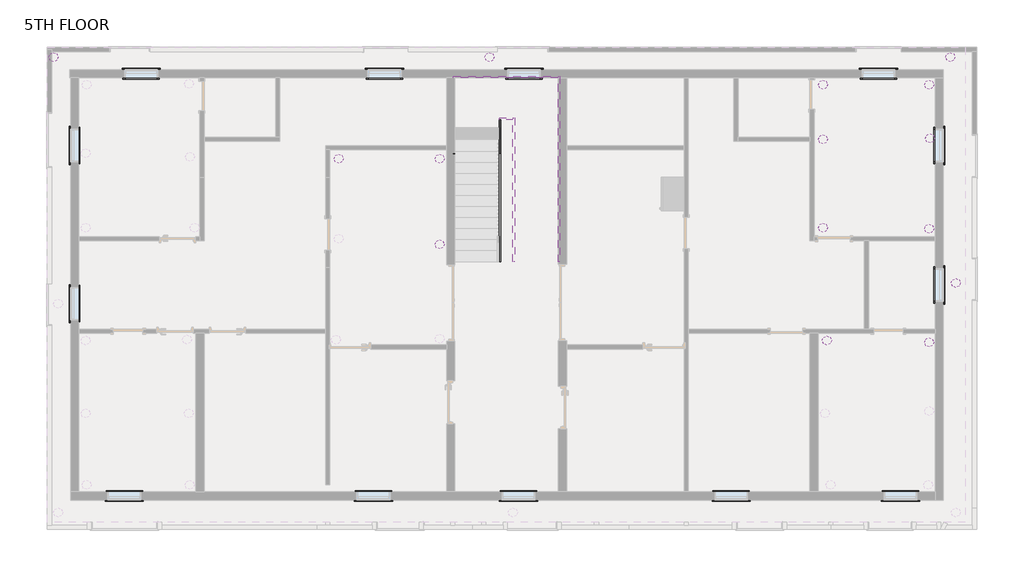
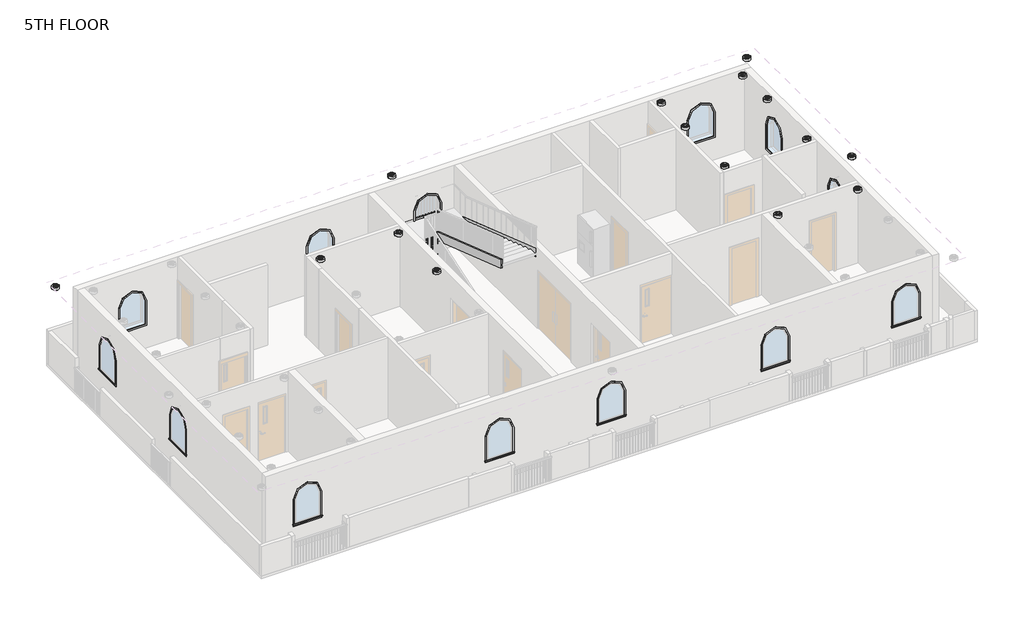
# One storey, part 7 of 7: 26 proxies, 15 light fixtures, 6 members.
"""IFC4 building model written with IfcOpenShell, lengths in millimetres."""

from ifc_helpers import new_model, si_unit, frame, origin, place, context, project, spatial, polyline, outline, extrude, transform, mapped, element, save
from components import trim_window_exterior_flat_arch_top_tree_centered_with_sill_aed3e54d, trim_window_interior_flat_arch_top_tree_centered_picture_e2e46177, ceiling_light_flat_round_60w_120v_7c4c2a52

model = new_model("IFC4")

# Units and contexts
model_context = context("Model", 3, world=origin())
ifc_project = project(units=[si_unit("LENGTHUNIT", "METRE", prefix="MILLI")], contexts=[model_context])

# Site, building, storey
site = spatial("IfcSite", under=ifc_project)
building = spatial("IfcBuilding", under=site)
storey = spatial("IfcBuildingStorey", under=building, Name="5TH FLOOR", Elevation=16002.0)

# Proxies
placement = place(None, origin())
trim_window_exterior_flat_arch_top_tree_centered_with_sill_shape = trim_window_exterior_flat_arch_top_tree_centered_with_sill_aed3e54d(model_context)
element("IfcBuildingElementProxy", 1, Name="Trim-Window-Exterior-Flat-Arch-Top-Tree_Centered : with Sill", ObjectType="Trim-Window-Exterior-Flat-Arch-Top-Tree_Centered : with Sill", at=placement, inside=storey, context=model_context, shape_type="MappedRepresentation", body=[
    mapped(trim_window_exterior_flat_arch_top_tree_centered_with_sill_shape, transform((-10967.3987925, -4014.0932193, 18288.0), x_axis=(1.0, 0.0, 0.0), y_axis=(0.0, 0.0, 1.0), z_axis=(0.0, -1.0, 0.0))),
])
element("IfcBuildingElementProxy", 2, Name="Trim-Window-Exterior-Flat-Arch-Top-Tree_Centered : with Sill", ObjectType="Trim-Window-Exterior-Flat-Arch-Top-Tree_Centered : with Sill", at=placement, inside=storey, context=model_context, shape_type="MappedRepresentation", body=[
    mapped(trim_window_exterior_flat_arch_top_tree_centered_with_sill_shape, transform((-4096.6987998, -4014.0932193, 18288.0), x_axis=(1.0, 0.0, 0.0), y_axis=(0.0, 0.0, 1.0), z_axis=(0.0, -1.0, 0.0))),
])
element("IfcBuildingElementProxy", 3, Name="Trim-Window-Exterior-Flat-Arch-Top-Tree_Centered : with Sill", ObjectType="Trim-Window-Exterior-Flat-Arch-Top-Tree_Centered : with Sill", at=placement, inside=storey, context=model_context, shape_type="MappedRepresentation", body=[
    mapped(trim_window_exterior_flat_arch_top_tree_centered_with_sill_shape, transform((-96.7067989, -4014.0932193, 18288.0), x_axis=(1.0, 0.0, 0.0), y_axis=(0.0, 0.0, 1.0), z_axis=(0.0, -1.0, 0.0))),
])
element("IfcBuildingElementProxy", 4, Name="Trim-Window-Exterior-Flat-Arch-Top-Tree_Centered : with Sill", ObjectType="Trim-Window-Exterior-Flat-Arch-Top-Tree_Centered : with Sill", at=placement, inside=storey, context=model_context, shape_type="MappedRepresentation", body=[
    mapped(trim_window_exterior_flat_arch_top_tree_centered_with_sill_shape, transform((5771.2012079, -4014.0932193, 18288.0), x_axis=(1.0, 0.0, 0.0), y_axis=(0.0, 0.0, 1.0), z_axis=(0.0, -1.0, 0.0))),
])
element("IfcBuildingElementProxy", 5, Name="Trim-Window-Exterior-Flat-Arch-Top-Tree_Centered : with Sill", ObjectType="Trim-Window-Exterior-Flat-Arch-Top-Tree_Centered : with Sill", at=placement, inside=storey, context=model_context, shape_type="MappedRepresentation", body=[
    mapped(trim_window_exterior_flat_arch_top_tree_centered_with_sill_shape, transform((10444.8012075, -4014.0932193, 18288.0), x_axis=(1.0, 0.0, 0.0), y_axis=(0.0, 0.0, 1.0), z_axis=(0.0, -1.0, 0.0))),
])
element("IfcBuildingElementProxy", 6, Name="Trim-Window-Exterior-Flat-Arch-Top-Tree_Centered : with Sill", ObjectType="Trim-Window-Exterior-Flat-Arch-Top-Tree_Centered : with Sill", at=placement, inside=storey, context=model_context, shape_type="MappedRepresentation", body=[
    mapped(trim_window_exterior_flat_arch_top_tree_centered_with_sill_shape, transform((11625.9012075, 1916.8067333, 18288.0), x_axis=(0.0, 1.0, 0.0), y_axis=(0.0, 0.0, 1.0), z_axis=(1.0, 0.0, 0.0))),
])
element("IfcBuildingElementProxy", 7, Name="Trim-Window-Exterior-Flat-Arch-Top-Tree_Centered : with Sill", ObjectType="Trim-Window-Exterior-Flat-Arch-Top-Tree_Centered : with Sill", at=placement, inside=storey, context=model_context, shape_type="MappedRepresentation", body=[
    mapped(trim_window_exterior_flat_arch_top_tree_centered_with_sill_shape, transform((11625.9012075, 5764.9067329, 18288.0), x_axis=(0.0, 1.0, 0.0), y_axis=(0.0, 0.0, 1.0), z_axis=(1.0, 0.0, 0.0))),
])
element("IfcBuildingElementProxy", 8, Name="Trim-Window-Exterior-Flat-Arch-Top-Tree_Centered : with Sill", ObjectType="Trim-Window-Exterior-Flat-Arch-Top-Tree_Centered : with Sill", at=placement, inside=storey, context=model_context, shape_type="MappedRepresentation", body=[
    mapped(trim_window_exterior_flat_arch_top_tree_centered_with_sill_shape, transform((9835.2012075, 7860.4067329, 18288.0), x_axis=(-1.0, 0.0, 0.0), y_axis=(0.0, 0.0, 1.0), z_axis=(0.0, 1.0, 0.0))),
])
element("IfcBuildingElementProxy", 9, Name="Trim-Window-Exterior-Flat-Arch-Top-Tree_Centered : with Sill", ObjectType="Trim-Window-Exterior-Flat-Arch-Top-Tree_Centered : with Sill", at=placement, inside=storey, context=model_context, shape_type="MappedRepresentation", body=[
    mapped(trim_window_exterior_flat_arch_top_tree_centered_with_sill_shape, transform((55.6932011, 7860.4067329, 18288.0), x_axis=(-1.0, 0.0, 0.0), y_axis=(0.0, 0.0, 1.0), z_axis=(0.0, 1.0, 0.0))),
])
element("IfcBuildingElementProxy", 10, Name="Trim-Window-Exterior-Flat-Arch-Top-Tree_Centered : with Sill", ObjectType="Trim-Window-Exterior-Flat-Arch-Top-Tree_Centered : with Sill", at=placement, inside=storey, context=model_context, shape_type="MappedRepresentation", body=[
    mapped(trim_window_exterior_flat_arch_top_tree_centered_with_sill_shape, transform((-3791.8987998, 7860.4067329, 18288.0), x_axis=(-1.0, 0.0, 0.0), y_axis=(0.0, 0.0, 1.0), z_axis=(0.0, 1.0, 0.0))),
])
element("IfcBuildingElementProxy", 11, Name="Trim-Window-Exterior-Flat-Arch-Top-Tree_Centered : with Sill", ObjectType="Trim-Window-Exterior-Flat-Arch-Top-Tree_Centered : with Sill", at=placement, inside=storey, context=model_context, shape_type="MappedRepresentation", body=[
    mapped(trim_window_exterior_flat_arch_top_tree_centered_with_sill_shape, transform((-10503.8487992, 7860.4067329, 18288.0), x_axis=(-1.0, 0.0, 0.0), y_axis=(0.0, 0.0, 1.0), z_axis=(0.0, 1.0, 0.0))),
])
element("IfcBuildingElementProxy", 12, Name="Trim-Window-Exterior-Flat-Arch-Top-Tree_Centered : with Sill", ObjectType="Trim-Window-Exterior-Flat-Arch-Top-Tree_Centered : with Sill", at=placement, inside=storey, context=model_context, shape_type="MappedRepresentation", body=[
    mapped(trim_window_exterior_flat_arch_top_tree_centered_with_sill_shape, transform((-12453.2987925, 5764.9067329, 18288.0), x_axis=(0.0, -1.0, 0.0), y_axis=(0.0, 0.0, 1.0), z_axis=(-1.0, 0.0, 0.0))),
])
element("IfcBuildingElementProxy", 13, Name="Trim-Window-Exterior-Flat-Arch-Top-Tree_Centered : with Sill", ObjectType="Trim-Window-Exterior-Flat-Arch-Top-Tree_Centered : with Sill", at=placement, inside=storey, context=model_context, shape_type="MappedRepresentation", body=[
    mapped(trim_window_exterior_flat_arch_top_tree_centered_with_sill_shape, transform((-12453.2987925, 1402.4567334, 18288.0), x_axis=(0.0, -1.0, 0.0), y_axis=(0.0, 0.0, 1.0), z_axis=(-1.0, 0.0, 0.0))),
])
trim_window_interior_flat_arch_top_tree_centered_picture_shape = trim_window_interior_flat_arch_top_tree_centered_picture_e2e46177(model_context)
element("IfcBuildingElementProxy", 14, Name="Trim-Window-Interior-Flat-Arch-Top-Tree_Centered : Picture Frame", ObjectType="Trim-Window-Interior-Flat-Arch-Top-Tree_Centered : Picture Frame", at=placement, inside=storey, context=model_context, shape_type="MappedRepresentation", body=[
    mapped(trim_window_interior_flat_arch_top_tree_centered_picture_shape, transform((-10967.3987925, -3785.4932193, 18288.0), x_axis=(-1.0, 0.0, 0.0), y_axis=(0.0, 0.0, 1.0), z_axis=(0.0, 1.0, 0.0))),
])
element("IfcBuildingElementProxy", 15, Name="Trim-Window-Interior-Flat-Arch-Top-Tree_Centered : Picture Frame", ObjectType="Trim-Window-Interior-Flat-Arch-Top-Tree_Centered : Picture Frame", at=placement, inside=storey, context=model_context, shape_type="MappedRepresentation", body=[
    mapped(trim_window_interior_flat_arch_top_tree_centered_picture_shape, transform((-4096.6987998, -3785.4932193, 18288.0), x_axis=(-1.0, 0.0, 0.0), y_axis=(0.0, 0.0, 1.0), z_axis=(0.0, 1.0, 0.0))),
])
element("IfcBuildingElementProxy", 16, Name="Trim-Window-Interior-Flat-Arch-Top-Tree_Centered : Picture Frame", ObjectType="Trim-Window-Interior-Flat-Arch-Top-Tree_Centered : Picture Frame", at=placement, inside=storey, context=model_context, shape_type="MappedRepresentation", body=[
    mapped(trim_window_interior_flat_arch_top_tree_centered_picture_shape, transform((-96.7067989, -3785.4932193, 18288.0), x_axis=(-1.0, 0.0, 0.0), y_axis=(0.0, 0.0, 1.0), z_axis=(0.0, 1.0, 0.0))),
])
element("IfcBuildingElementProxy", 17, Name="Trim-Window-Interior-Flat-Arch-Top-Tree_Centered : Picture Frame", ObjectType="Trim-Window-Interior-Flat-Arch-Top-Tree_Centered : Picture Frame", at=placement, inside=storey, context=model_context, shape_type="MappedRepresentation", body=[
    mapped(trim_window_interior_flat_arch_top_tree_centered_picture_shape, transform((5771.2012079, -3785.4932193, 18288.0), x_axis=(-1.0, 0.0, 0.0), y_axis=(0.0, 0.0, 1.0), z_axis=(0.0, 1.0, 0.0))),
])
element("IfcBuildingElementProxy", 18, Name="Trim-Window-Interior-Flat-Arch-Top-Tree_Centered : Picture Frame", ObjectType="Trim-Window-Interior-Flat-Arch-Top-Tree_Centered : Picture Frame", at=placement, inside=storey, context=model_context, shape_type="MappedRepresentation", body=[
    mapped(trim_window_interior_flat_arch_top_tree_centered_picture_shape, transform((10444.8012075, -3785.4932193, 18288.0), x_axis=(-1.0, 0.0, 0.0), y_axis=(0.0, 0.0, 1.0), z_axis=(0.0, 1.0, 0.0))),
])
element("IfcBuildingElementProxy", 19, Name="Trim-Window-Interior-Flat-Arch-Top-Tree_Centered : Picture Frame", ObjectType="Trim-Window-Interior-Flat-Arch-Top-Tree_Centered : Picture Frame", at=placement, inside=storey, context=model_context, shape_type="MappedRepresentation", body=[
    mapped(trim_window_interior_flat_arch_top_tree_centered_picture_shape, transform((11397.3012075, 1916.8067333, 18288.0), x_axis=(0.0, -1.0, 0.0), y_axis=(0.0, 0.0, 1.0), z_axis=(-1.0, 0.0, 0.0))),
])
element("IfcBuildingElementProxy", 20, Name="Trim-Window-Interior-Flat-Arch-Top-Tree_Centered : Picture Frame", ObjectType="Trim-Window-Interior-Flat-Arch-Top-Tree_Centered : Picture Frame", at=placement, inside=storey, context=model_context, shape_type="MappedRepresentation", body=[
    mapped(trim_window_interior_flat_arch_top_tree_centered_picture_shape, transform((11397.3012075, 5764.9067329, 18288.0), x_axis=(0.0, -1.0, 0.0), y_axis=(0.0, 0.0, 1.0), z_axis=(-1.0, 0.0, 0.0))),
])
element("IfcBuildingElementProxy", 21, Name="Trim-Window-Interior-Flat-Arch-Top-Tree_Centered : Picture Frame", ObjectType="Trim-Window-Interior-Flat-Arch-Top-Tree_Centered : Picture Frame", at=placement, inside=storey, context=model_context, shape_type="MappedRepresentation", body=[
    mapped(trim_window_interior_flat_arch_top_tree_centered_picture_shape, transform((9835.2012075, 7631.8067329, 18288.0), x_axis=(1.0, 0.0, 0.0), y_axis=(0.0, 0.0, 1.0), z_axis=(0.0, -1.0, 0.0))),
])
element("IfcBuildingElementProxy", 22, Name="Trim-Window-Interior-Flat-Arch-Top-Tree_Centered : Picture Frame", ObjectType="Trim-Window-Interior-Flat-Arch-Top-Tree_Centered : Picture Frame", at=placement, inside=storey, context=model_context, shape_type="MappedRepresentation", body=[
    mapped(trim_window_interior_flat_arch_top_tree_centered_picture_shape, transform((55.6932011, 7631.8067329, 18288.0), x_axis=(1.0, 0.0, 0.0), y_axis=(0.0, 0.0, 1.0), z_axis=(0.0, -1.0, 0.0))),
])
element("IfcBuildingElementProxy", 23, Name="Trim-Window-Interior-Flat-Arch-Top-Tree_Centered : Picture Frame", ObjectType="Trim-Window-Interior-Flat-Arch-Top-Tree_Centered : Picture Frame", at=placement, inside=storey, context=model_context, shape_type="MappedRepresentation", body=[
    mapped(trim_window_interior_flat_arch_top_tree_centered_picture_shape, transform((-3791.8987998, 7631.8067329, 18288.0), x_axis=(1.0, 0.0, 0.0), y_axis=(0.0, 0.0, 1.0), z_axis=(0.0, -1.0, 0.0))),
])
element("IfcBuildingElementProxy", 24, Name="Trim-Window-Interior-Flat-Arch-Top-Tree_Centered : Picture Frame", ObjectType="Trim-Window-Interior-Flat-Arch-Top-Tree_Centered : Picture Frame", at=placement, inside=storey, context=model_context, shape_type="MappedRepresentation", body=[
    mapped(trim_window_interior_flat_arch_top_tree_centered_picture_shape, transform((-10503.8487992, 7631.8067329, 18288.0), x_axis=(1.0, 0.0, 0.0), y_axis=(0.0, 0.0, 1.0), z_axis=(0.0, -1.0, 0.0))),
])
element("IfcBuildingElementProxy", 25, Name="Trim-Window-Interior-Flat-Arch-Top-Tree_Centered : Picture Frame", ObjectType="Trim-Window-Interior-Flat-Arch-Top-Tree_Centered : Picture Frame", at=placement, inside=storey, context=model_context, shape_type="MappedRepresentation", body=[
    mapped(trim_window_interior_flat_arch_top_tree_centered_picture_shape, transform((-12224.6987925, 5764.9067329, 18288.0), x_axis=(0.0, 1.0, 0.0), y_axis=(0.0, 0.0, 1.0), z_axis=(1.0, 0.0, 0.0))),
])
element("IfcBuildingElementProxy", 26, Name="Trim-Window-Interior-Flat-Arch-Top-Tree_Centered : Picture Frame", ObjectType="Trim-Window-Interior-Flat-Arch-Top-Tree_Centered : Picture Frame", at=placement, inside=storey, context=model_context, shape_type="MappedRepresentation", body=[
    mapped(trim_window_interior_flat_arch_top_tree_centered_picture_shape, transform((-12224.6987925, 1402.4567334, 18288.0), x_axis=(0.0, 1.0, 0.0), y_axis=(0.0, 0.0, 1.0), z_axis=(1.0, 0.0, 0.0))),
])

# Light fixtures
ceiling_light_flat_round_60w_120v_shape = ceiling_light_flat_round_60w_120v_7c4c2a52(model_context)
element("IfcLightFixture", 27, ObjectType="Ceiling Light - Flat Round : 60W - 120V", at=placement, inside=storey, context=model_context, shape_type="MappedRepresentation", body=[
    mapped(ceiling_light_flat_round_60w_120v_shape, transform((-12923.1987925, 8203.3067329, 16611.6), x_axis=(1.0, 0.0, 0.0), y_axis=(0.0, 1.0, 0.0), z_axis=(0.0, 0.0, 1.0))),
])
element("IfcLightFixture", 28, ObjectType="Ceiling Light - Flat Round : 60W - 120V", at=placement, inside=storey, context=model_context, shape_type="MappedRepresentation", body=[
    mapped(ceiling_light_flat_round_60w_120v_shape, transform((-896.2987998, 8203.3067329, 16611.6), x_axis=(1.0, 0.0, 0.0), y_axis=(0.0, 1.0, 0.0), z_axis=(0.0, 0.0, 1.0))),
])
element("IfcLightFixture", 29, ObjectType="Ceiling Light - Flat Round : 60W - 120V", at=placement, inside=storey, context=model_context, shape_type="MappedRepresentation", body=[
    mapped(ceiling_light_flat_round_60w_120v_shape, transform((11816.4012075, 8203.3067329, 16611.6), x_axis=(1.0, 0.0, 0.0), y_axis=(0.0, 1.0, 0.0), z_axis=(0.0, 0.0, 1.0))),
])
element("IfcLightFixture", 30, ObjectType="Ceiling Light - Flat Round : 60W - 120V", at=placement, inside=storey, context=model_context, shape_type="MappedRepresentation", body=[
    mapped(ceiling_light_flat_round_60w_120v_shape, transform((11968.8012075, 1973.9567332, 16611.6), x_axis=(1.0, 0.0, 0.0), y_axis=(0.0, 1.0, 0.0), z_axis=(0.0, 0.0, 1.0))),
])
element("IfcLightFixture", 31, ObjectType="Ceiling Light - Flat Round : 60W - 120V", at=placement, inside=storey, context=model_context, shape_type="MappedRepresentation", body=[
    mapped(ceiling_light_flat_round_60w_120v_shape, transform((8304.8512079, 7441.3067329, 16611.6), x_axis=(1.0, 0.0, 0.0), y_axis=(0.0, 1.0, 0.0), z_axis=(0.0, 0.0, 1.0))),
])
element("IfcLightFixture", 32, ObjectType="Ceiling Light - Flat Round : 60W - 120V", at=placement, inside=storey, context=model_context, shape_type="MappedRepresentation", body=[
    mapped(ceiling_light_flat_round_60w_120v_shape, transform((11232.2012075, 7441.3067329, 16611.6), x_axis=(1.0, 0.0, 0.0), y_axis=(0.0, 1.0, 0.0), z_axis=(0.0, 0.0, 1.0))),
])
element("IfcLightFixture", 33, ObjectType="Ceiling Light - Flat Round : 60W - 120V", at=placement, inside=storey, context=model_context, shape_type="MappedRepresentation", body=[
    mapped(ceiling_light_flat_round_60w_120v_shape, transform((8304.8512079, 3497.9567332, 16611.6), x_axis=(1.0, 0.0, 0.0), y_axis=(0.0, 1.0, 0.0), z_axis=(0.0, 0.0, 1.0))),
])
element("IfcLightFixture", 34, ObjectType="Ceiling Light - Flat Round : 60W - 120V", at=placement, inside=storey, context=model_context, shape_type="MappedRepresentation", body=[
    mapped(ceiling_light_flat_round_60w_120v_shape, transform((11232.2012075, 3472.5567332, 16611.6), x_axis=(1.0, 0.0, 0.0), y_axis=(0.0, 1.0, 0.0), z_axis=(0.0, 0.0, 1.0))),
])
element("IfcLightFixture", 35, ObjectType="Ceiling Light - Flat Round : 60W - 120V", at=placement, inside=storey, context=model_context, shape_type="MappedRepresentation", body=[
    mapped(ceiling_light_flat_round_60w_120v_shape, transform((8412.8012079, 386.4567334, 16611.6), x_axis=(1.0, 0.0, 0.0), y_axis=(0.0, 1.0, 0.0), z_axis=(0.0, 0.0, 1.0))),
])
element("IfcLightFixture", 36, ObjectType="Ceiling Light - Flat Round : 60W - 120V", at=placement, inside=storey, context=model_context, shape_type="MappedRepresentation", body=[
    mapped(ceiling_light_flat_round_60w_120v_shape, transform((11232.2012075, 335.6567334, 16611.6), x_axis=(1.0, 0.0, 0.0), y_axis=(0.0, 1.0, 0.0), z_axis=(0.0, 0.0, 1.0))),
])
element("IfcLightFixture", 37, ObjectType="Ceiling Light - Flat Round : 60W - 120V", at=placement, inside=storey, context=model_context, shape_type="MappedRepresentation", body=[
    mapped(ceiling_light_flat_round_60w_120v_shape, transform((-5055.5487995, 5402.9567329, 16611.6), x_axis=(1.0, 0.0, 0.0), y_axis=(0.0, 1.0, 0.0), z_axis=(0.0, 0.0, 1.0))),
])
element("IfcLightFixture", 38, ObjectType="Ceiling Light - Flat Round : 60W - 120V", at=placement, inside=storey, context=model_context, shape_type="MappedRepresentation", body=[
    mapped(ceiling_light_flat_round_60w_120v_shape, transform((-2267.8987998, 5402.9567329, 16611.6), x_axis=(1.0, 0.0, 0.0), y_axis=(0.0, 1.0, 0.0), z_axis=(0.0, 0.0, 1.0))),
])
element("IfcLightFixture", 39, ObjectType="Ceiling Light - Flat Round : 60W - 120V", at=placement, inside=storey, context=model_context, shape_type="MappedRepresentation", body=[
    mapped(ceiling_light_flat_round_60w_120v_shape, transform((8304.8512079, 5936.3567329, 16611.6), x_axis=(1.0, 0.0, 0.0), y_axis=(0.0, 1.0, 0.0), z_axis=(0.0, 0.0, 1.0))),
])
element("IfcLightFixture", 40, ObjectType="Ceiling Light - Flat Round : 60W - 120V", at=placement, inside=storey, context=model_context, shape_type="MappedRepresentation", body=[
    mapped(ceiling_light_flat_round_60w_120v_shape, transform((11257.6012075, 5961.7567329, 16611.6), x_axis=(1.0, 0.0, 0.0), y_axis=(0.0, 1.0, 0.0), z_axis=(0.0, 0.0, 1.0))),
])
element("IfcLightFixture", 41, ObjectType="Ceiling Light - Flat Round : 60W - 120V", at=placement, inside=storey, context=model_context, shape_type="MappedRepresentation", body=[
    mapped(ceiling_light_flat_round_60w_120v_shape, transform((-2267.8987998, 3040.7567332, 16611.6), x_axis=(1.0, 0.0, 0.0), y_axis=(0.0, 1.0, 0.0), z_axis=(0.0, 0.0, 1.0))),
])

# Members
element("IfcMember", 42, ObjectType="Stringer - 2\" Width", at=placement, inside=storey, context=model_context, shape_type="SweptSolid", body=[
    extrude(outline(polyline([(2564.5067329, 16002.0), (2564.5067329, 16195.238056), (6486.7524627, 17526.0), (7435.4093802, 17526.0), (2943.6199065, 16002.0), (2564.5067329, 16002.0)])), frame((-1899.5987998, 0.0, 0.0), z_axis=(1.0, 0.0, 0.0), x_axis=(0.0, 1.0, 0.0)), (0.0, 0.0, 1.0), 50.8),
])
element("IfcMember", 43, ObjectType="Stringer - 2\" Width", at=placement, inside=storey, context=model_context, shape_type="SweptSolid", body=[
    extrude(outline(polyline([(-1899.5987998, 7631.8067329), (-1899.5987998, 7682.6067329), (996.0012002, 7682.6067329), (996.0012002, 7631.8067329), (-1899.5987998, 7631.8067329)])), frame((0.0, 0.0, 17221.2), z_axis=(0.0, 0.0, 1.0), x_axis=(1.0, 0.0, 0.0)), (0.0, 0.0, 1.0), 304.8),
])
element("IfcMember", 44, ObjectType="Stringer - 2\" Width", at=placement, inside=storey, context=model_context, shape_type="SweptSolid", body=[
    extrude(outline(polyline([(7682.6067329, 17250.925556), (7682.6067329, 17221.2), (6821.5619804, 17221.2), (2564.5067329, 18665.5580304), (2564.5067329, 18987.4237702), (7682.6067329, 17250.925556)])), frame((996.0012002, 0.0, 0.0), z_axis=(1.0, 0.0, 0.0), x_axis=(0.0, 1.0, 0.0)), (0.0, 0.0, 1.0), 50.8),
])
element("IfcMember", 45, ObjectType="Stringer - 2\" Width", at=placement, inside=storey, context=model_context, shape_type="SweptSolid", body=[
    extrude(outline(polyline([(2564.5067329, 16002.0), (2564.5067329, 16195.238056), (6476.1067329, 17522.388056), (6476.1067329, 17200.5223161), (2943.6199065, 16002.0), (2564.5067329, 16002.0)])), frame((-629.5987998, 0.0, 0.0), z_axis=(1.0, 0.0, 0.0), x_axis=(0.0, 1.0, 0.0)), (0.0, 0.0, 1.0), 50.8),
])
element("IfcMember", 46, ObjectType="Stringer - 2\" Width", at=placement, inside=storey, context=model_context, shape_type="SweptSolid", body=[
    extrude(outline(polyline([(-629.5987998, 6476.1067329), (-629.5987998, 6526.9067329), (-248.5987915, 6526.9067329), (-248.5987915, 6476.1067329), (-629.5987998, 6476.1067329)])), frame((0.0, 0.0, 17221.2), z_axis=(0.0, 0.0, 1.0), x_axis=(1.0, 0.0, 0.0)), (0.0, 0.0, 1.0), 304.8),
])
element("IfcMember", 47, ObjectType="Stringer - 2\" Width", at=placement, inside=storey, context=model_context, shape_type="SweptSolid", body=[
    extrude(outline(polyline([(6526.9067329, 17643.038056), (6526.9067329, 17321.1723161), (2564.5067329, 18665.5580304), (2564.5067329, 18987.4237702), (6526.9067329, 17643.038056)])), frame((-248.5987915, 0.0, 0.0), z_axis=(1.0, 0.0, 0.0), x_axis=(0.0, 1.0, 0.0)), (0.0, 0.0, 1.0), 50.8),
])

save(model, "model.ifc")

# Revit data of these elements
# Type "Trim-Window-Exterior-Flat-Arch-Top-Tree_Centered : with Sill"
#   Trim Width = 0' - 2 1/4"
#   Trim Thickness_Picture Frame = 0' - 1 1/4"
#   Trim Thickness_with Sill = 0' - 0 3/4"
#   Sill Thickness = 0' - 1 1/4"
#   Opening Width [instance default] = 2' - 0"
#   Opening Height [instance default] = 3' - 0"
#   Default Elevation = 4' - 0"
#   Sill = yes
#   Picture Frame = no
#   Trim Material [instance default] = none
# Type "Trim-Window-Interior-Flat-Arch-Top-Tree_Centered : Picture Frame"
#   Trim Thickness_Picture Frame = 0' - 1 1/4"
#   Trim Width = 0' - 2 1/4"
#   Trim Thickness_with Sill = 0' - 0 3/4"
#   Sill Thickness = 0' - 1 1/4"
#   Opening Width [instance default] = 2' - 0"
#   Opening Height [instance default] = 3' - 0"
#   Default Elevation = 4' - 0"
#   Sill = no
#   Picture Frame = yes
#   Trim Material [instance default] = none
# Type "Ceiling Light - Flat Round : 60W - 120V"
#   Lamp = "A-19"
#   Assembly Code = "D5020220"
#   Wattage = 60 W
#   built-in parameter 1150110 = 1 (stored number, unit not read)
#   built-in parameter 1114217 = 1 (stored number, unit not read)
#   built-in parameter 1150109 = 1 (stored number, unit not read)
#   built-in parameter 1150113 = 1 (stored number, unit not read)
#   built-in parameter 1150115 = 1 (stored number, unit not read)
#   built-in parameter 1150105 = 272.155 (stored number, unit not read)
#   Light Source Symbol Size = 2' - 0"
#   built-in parameter 1150112 = 1 (stored number, unit not read)
#   built-in parameter 1150114 = 1 (stored number, unit not read)
#   built-in parameter 1150107 = 2800 (stored number, unit not read)
#   built-in parameter 1150106 = 2.72155 (stored number, unit not read)
#   Emit from Circle Diameter = 0' - 10"
#   built-in parameter 1150104 = 1.32387 (stored number, unit not read)
#   Ballast Voltage = 120 V
#   built-in parameter 1114218 = 1 (stored number, unit not read)
#   built-in parameter 1150133 = 10 (stored number, unit not read)
#   Lumens = 855 lm
#   Apparent Load = 60 VA
#   built-in parameter 1150134 = 4
#   built-in parameter 1150137 = 1
#   Color Filter = 16777215
#   built-in parameter 1140040 [instance default] = 1
#   Ballast Number of Poles = 1
#   Light Box Material = Steel, Paint Finish, Dark Gray, Matte
#   Diffuser Material = Glass, White, High Luminance
#   Wattage Comments = ""
#   Emit Shape Visible in Rendering = no
#   Dimming Lamp Color Temperature Shift = (empty or 0)
#   Default Elevation = 0
# Elements 1, 2, 3, 4, 5, 6, 7, 8, 9, 10, 11, 12, 13 (IfcBuildingElementProxy, "Trim-Window-Exterior-Flat-Arch-Top-Tree_Centered : with Sill")
#   Opening Width = 3' - 0"
#   Opening Height = 4' - 6"
#   Trim Material = Clad - White
#   Phase Created = New Construction
#   Materials on its faces: "Clad - White"
# Elements 14, 15, 16, 17, 18, 19, 20, 21, 22, 23, 24, 25, 26 (IfcBuildingElementProxy, "Trim-Window-Interior-Flat-Arch-Top-Tree_Centered : Picture Frame")
#   Opening Width = 3' - 0"
#   Opening Height = 4' - 6"
#   Trim Material = Wood - Stained
#   Phase Created = New Construction
#   Materials on its faces: "Wood - Stained"
# Element 27 (IfcLightFixture, "Ceiling Light - Flat Round : 60W - 120V")
#   Mark = "136"
#   built-in parameter 1140040 = 1
#   Phase Created = New Construction
#   Materials on its faces: "Glass, White, High Luminance", "Steel, Paint Finish, Dark Gray, Matte"
# Element 28 (IfcLightFixture, "Ceiling Light - Flat Round : 60W - 120V")
#   Mark = "137"
#   built-in parameter 1140040 = 1
#   Phase Created = New Construction
#   Materials on its faces: "Glass, White, High Luminance", "Steel, Paint Finish, Dark Gray, Matte"
# Element 29 (IfcLightFixture, "Ceiling Light - Flat Round : 60W - 120V")
#   Mark = "138"
#   built-in parameter 1140040 = 1
#   Phase Created = New Construction
#   Materials on its faces: "Glass, White, High Luminance", "Steel, Paint Finish, Dark Gray, Matte"
# Element 30 (IfcLightFixture, "Ceiling Light - Flat Round : 60W - 120V")
#   Mark = "142"
#   built-in parameter 1140040 = 1
#   Phase Created = New Construction
#   Materials on its faces: "Glass, White, High Luminance", "Steel, Paint Finish, Dark Gray, Matte"
# Element 31 (IfcLightFixture, "Ceiling Light - Flat Round : 60W - 120V")
#   Mark = "152"
#   built-in parameter 1140040 = 1
#   Phase Created = New Construction
#   Materials on its faces: "Glass, White, High Luminance", "Steel, Paint Finish, Dark Gray, Matte"
# Element 32 (IfcLightFixture, "Ceiling Light - Flat Round : 60W - 120V")
#   Mark = "153"
#   built-in parameter 1140040 = 1
#   Phase Created = New Construction
#   Materials on its faces: "Glass, White, High Luminance", "Steel, Paint Finish, Dark Gray, Matte"
# Element 33 (IfcLightFixture, "Ceiling Light - Flat Round : 60W - 120V")
#   Mark = "154"
#   built-in parameter 1140040 = 1
#   Phase Created = New Construction
#   Materials on its faces: "Glass, White, High Luminance", "Steel, Paint Finish, Dark Gray, Matte"
# Element 34 (IfcLightFixture, "Ceiling Light - Flat Round : 60W - 120V")
#   Mark = "155"
#   built-in parameter 1140040 = 1
#   Phase Created = New Construction
#   Materials on its faces: "Glass, White, High Luminance", "Steel, Paint Finish, Dark Gray, Matte"
# Element 35 (IfcLightFixture, "Ceiling Light - Flat Round : 60W - 120V")
#   Mark = "156"
#   built-in parameter 1140040 = 1
#   Phase Created = New Construction
#   Materials on its faces: "Glass, White, High Luminance", "Steel, Paint Finish, Dark Gray, Matte"
# Element 36 (IfcLightFixture, "Ceiling Light - Flat Round : 60W - 120V")
#   Mark = "157"
#   built-in parameter 1140040 = 1
#   Phase Created = New Construction
#   Materials on its faces: "Glass, White, High Luminance", "Steel, Paint Finish, Dark Gray, Matte"
# Element 37 (IfcLightFixture, "Ceiling Light - Flat Round : 60W - 120V")
#   Mark = "160"
#   built-in parameter 1140040 = 1
#   Phase Created = New Construction
#   Materials on its faces: "Glass, White, High Luminance", "Steel, Paint Finish, Dark Gray, Matte"
# Element 38 (IfcLightFixture, "Ceiling Light - Flat Round : 60W - 120V")
#   Mark = "161"
#   built-in parameter 1140040 = 1
#   Phase Created = New Construction
#   Materials on its faces: "Glass, White, High Luminance", "Steel, Paint Finish, Dark Gray, Matte"
# Element 39 (IfcLightFixture, "Ceiling Light - Flat Round : 60W - 120V")
#   Mark = "166"
#   built-in parameter 1140040 = 1
#   Phase Created = New Construction
#   Materials on its faces: "Glass, White, High Luminance", "Steel, Paint Finish, Dark Gray, Matte"
# Element 40 (IfcLightFixture, "Ceiling Light - Flat Round : 60W - 120V")
#   Mark = "167"
#   built-in parameter 1140040 = 1
#   Phase Created = New Construction
#   Materials on its faces: "Glass, White, High Luminance", "Steel, Paint Finish, Dark Gray, Matte"
# Element 41 (IfcLightFixture, "Ceiling Light - Flat Round : 60W - 120V")
#   Mark = "169"
#   built-in parameter 1140040 = 1
#   Phase Created = New Construction
#   Materials on its faces: "Glass, White, High Luminance", "Steel, Paint Finish, Dark Gray, Matte"
# Elements 42, 43, 44, 45, 46, 47 (IfcMember, "Stringer - 2\" Width")
#   Phase Created = New Construction
# Materials
#   "Steel, Paint Finish, Dark Gray, Matte": class "Metal", colour RGB 98 98 98, transparency 0, Description = "Steel, paint finish, dark gray, matte", Cost = 0
#   "Glass, White, High Luminance": class "Glass", colour RGB 249 250 249, transparency 0.8, Description = "physical material", Cost = 0
#   "Clad - White": class "Wood", colour RGB 242 242 238, transparency 0, Cost = 0
#   "Wood - Stained": class "Wood", colour RGB 224 178 126, transparency 0, Cost = 0
